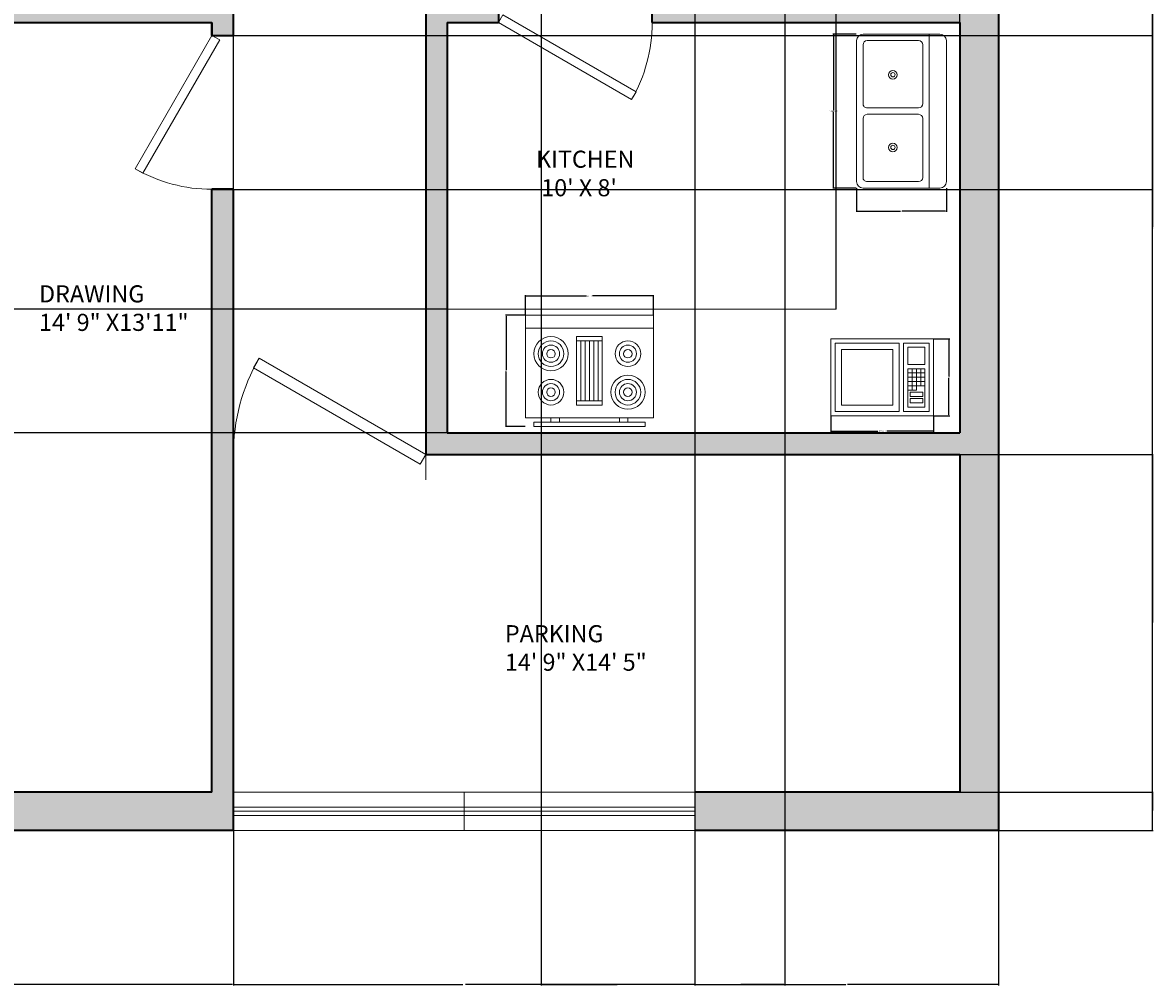
# Model space of a CAD drawing. Units: inches. Extents: x -29 to 404, y -32 to 761.
# Tile 2 of 5: x 139 to 404, y -32 to 193. Entities that reach past the tile are written whole.
import ezdxf

# ---------------------------------------------------------------- set-up
doc = ezdxf.new("R2010")
doc.units = ezdxf.units.IN
doc.header["$MEASUREMENT"] = 0
for name, color, linetype, lineweight in [('A-ANNO-DIMS', 2, 'Continuous', 18), ('A-AREA-IDEN', 7, 'Continuous', 18), ('A-EQPM', 8, 'Continuous', 18), ('A-FLOR-CASE', 8, 'Continuous', 20), ('A-FLOR-FIXT', 9, 'Continuous', 18), ('A-WALL', 7, 'Continuous', 35), ('doors', 40, 'Continuous', 20)]:
    doc.layers.add(name, color=color, linetype=linetype, lineweight=lineweight)
doc.layers.add('A-WALL-PATT', color=251, linetype='Continuous', lineweight=13, true_color=0x636466)
doc.styles.get("Standard").update_dxf_attribs({"font": 'arial.ttf'})
doc.dimstyles.get("Standard").update_dxf_attribs({"dimtxt": 0.18, "dimasz": 0.18, "dimexe": 0.18, "dimexo": 0.0625, "dimgap": 0.09, "dimtad": 0, "dimtih": 1, "dimtoh": 1, "dimdec": 4, "dimzin": 0, "dimdsep": 46, "dimtxsty": 'Standard', "dimcen": 0.09, "dimadec": 0, "dimazin": 0, "dimtfac": 1, "dimtdec": 4, "dimtofl": 0, "dimtmove": 0, "dimatfit": 3, "dimfxl": 1, "dimtolj": 1, "dimtzin": 0, "dimarcsym": 0})

# ---------------------------------------------------------------- blocks, each defined once
blk = doc.blocks.new('Range-Oven - 30 in top')
for p, q in [((0, -3), (30, -3)), ((12, -6), (18, -6)), ((13, -20), (13, -6)), ((14, -6), (14, -20)), ((15, -20), (15, -6)), ((16, -6), (16, -20)), ((17, -20), (17, -6)), ((18, -20), (12, -20)), ((6, -24), (6, -25)), ((8, -25), (8, -24)), ((22, -25), (22, -24)), ((24, -24), (24, -25))]:
    blk.add_line(p, q)
for points in [[(0, -24), (0, 0), (30, 0), (30, -24)], [(12, -21), (12, -5), (18, -5), (18, -21)], [(2, -26), (2, -25), (28, -25), (28, -26)]]:
    blk.add_lwpolyline(points, close=True)
for centre, radius in [((6, -9), 4), ((6, -9), 3), ((6, -9), 2), ((24, -9), 3), ((24, -9), 2), ((6, -9), 1), ((24, -9), 1), ((6, -18), 3), ((24, -18), 4), ((24, -18), 3), ((6, -18), 2), ((6, -18), 1), ((24, -18), 2), ((24, -18), 1)]:
    blk.add_circle(centre, radius)
blk = doc.blocks.new('Sink-double - 36 in top')
for p, q in [((-18, -4), (18, -4)), ((-0.75, -18.5), (-0.75, -6.5)), ((0.75, -6.5), (0.75, -18.5))]:
    blk.add_line(p, q)
for points in [[(-16.5, 0), (16.5, 0)], [(-18, -19.5), (-18, -1.5)], [(18, -1.5), (18, -19.5)], [(-16.5, -18.5), (-16.5, -6.5)], [(-15.5, -5.5), (-1.75, -5.5)], [(1.75, -5.5), (15.5, -5.5)], [(16.5, -6.5), (16.5, -18.5)], [(16.5, -21), (-16.5, -21)], [(-1.75, -19.5), (-15.5, -19.5)], [(15.5, -19.5), (1.75, -19.5)]]:
    blk.add_lwpolyline(points)
for centre, radius in [((-8.5, -12.5), 1), ((-8.5, -12.5), 0.5), ((8.5, -12.5), 1), ((8.5, -12.5), 0.5)]:
    blk.add_circle(centre, radius)
for centre, radius, start, end in [((-16.5, -1.5), 1.5, 90, 180), ((16.5, -1.5), 1.5, 0, 90), ((-15.5, -6.5), 1, 90, 180), ((-1.75, -6.5), 1, 0, 90), ((1.75, -6.5), 1, 90, 180), ((15.5, -6.5), 1, 0, 90), ((-15.5, -18.5), 1, 180, 270), ((-1.75, -18.5), 1, 270, 0), ((1.75, -18.5), 1, 180, 270), ((15.5, -18.5), 1, 270, 0), ((-16.5, -19.5), 1.5, 180, 270), ((16.5, -19.5), 1.5, 270, 0)]:
    blk.add_arc(centre, radius, start, end)
blk = doc.blocks.new('Microwave')
for p, q in [((19, 7), (19, 11)), ((20, 11), (20, 7)), ((21, 7), (21, 11)), ((18, 10), (22, 10)), ((22, 9), (18, 9)), ((18, 8), (22, 8)), ((22, 7), (18, 7)), ((20, 6), (18, 6)), ((19, 6), (19, 7)), ((20, 7), (20, 6))]:
    blk.add_line(p, q)
for points in [[(0, 0), (0, 18), (24, 18), (24, 0)], [(1, 1), (1, 17), (16, 17), (16, 1)], [(17, 1), (17, 17), (23, 17), (23, 1)], [(18, 12), (18, 16), (22, 16), (22, 12)], [(2.5, 2.5), (2.5, 15.5), (14.5, 15.5), (14.5, 2.5)], [(18, 2), (18, 11), (22, 11), (22, 2)], [(18.5, 4.5), (18.5, 5.5), (21.5, 5.5), (21.5, 4.5)], [(18.5, 3), (18.5, 4), (21.5, 4), (21.5, 3)]]:
    blk.add_lwpolyline(points, close=True)
blk = doc.blocks.new('*U7')
for p, q in [((0, 0), (0, 100)), ((750, 0), (750, 100))]:
    blk.add_line(p, q)
blk.add_lwpolyline([(0, 0), (649.5, -375), (671.4, -337.1), (21.9, 37.9)], close=True)
blk.add_arc((0, 0), 750, 330, 0)
blk = doc.blocks.new('*D25')
at = {"layer": 'A-ANNO-DIMS', "color": 0, "lineweight": -2, "transparency": 16777216}
for p, q in [((256.99, 125.04), (256.99, 129.66)), ((286.99, 125.04), (286.99, 129.66)), ((257.17, 129.48), (271.3, 129.48)), ((286.81, 129.48), (272.69, 129.48))]:
    blk.add_line(p, q, dxfattribs=at)
at = {"layer": 'A-ANNO-DIMS', "color": 0, "transparency": 16777216}
for points in [[(257.17, 129.51), (257.17, 129.45), (256.99, 129.48)], [(286.81, 129.51), (286.81, 129.45), (286.99, 129.48)]]:
    blk.add_solid(points, dxfattribs=at)
at = {"layer": 'Defpoints', "color": 0, "transparency": 16777216}
for p in [(286.99, 129.48), (256.99, 124.98), (286.99, 124.98)]:
    blk.add_point(p, dxfattribs=at)
at = {"layer": 'A-ANNO-DIMS', "color": 0, "transparency": 16777216, "insert": (271.99, 129.48), "char_height": 0.18, "attachment_point": 5}
blk.add_mtext('\\A1;RANGE 30', dxfattribs=at)
blk = doc.blocks.new('*D26')
at = {"layer": 'A-ANNO-DIMS', "color": 0, "lineweight": -2, "transparency": 16777216}
for p, q in [((256.93, 124.98), (252.31, 124.98)), ((252.49, 124.8), (252.49, 112.16)), ((252.49, 99.16), (252.49, 111.8)), ((256.93, 98.98), (252.31, 98.98))]:
    blk.add_line(p, q, dxfattribs=at)
at = {"layer": 'A-ANNO-DIMS', "color": 0, "transparency": 16777216}
for points in [[(252.46, 124.8), (252.52, 124.8), (252.49, 124.98)], [(252.46, 99.16), (252.52, 99.16), (252.49, 98.98)]]:
    blk.add_solid(points, dxfattribs=at)
at = {"layer": 'Defpoints', "color": 0, "transparency": 16777216}
for p in [(252.49, 124.98), (256.99, 124.98), (256.99, 98.98)]:
    blk.add_point(p, dxfattribs=at)
at = {"layer": 'A-ANNO-DIMS', "color": 0, "transparency": 16777216, "insert": (252.49, 111.98), "char_height": 0.18, "attachment_point": 5}
blk.add_mtext('\\A1;26', dxfattribs=at)
blk = doc.blocks.new('*D27')
at = {"layer": 'A-ANNO-DIMS', "color": 0, "lineweight": -2, "transparency": 16777216}
for p, q in [((334.43, 190.73), (328.91, 190.73)), ((329.09, 190.55), (329.09, 172.91)), ((329.09, 154.91), (329.09, 172.55)), ((334.43, 154.73), (328.91, 154.73))]:
    blk.add_line(p, q, dxfattribs=at)
at = {"layer": 'A-ANNO-DIMS', "color": 0, "transparency": 16777216}
for points in [[(329.06, 190.55), (329.12, 190.55), (329.09, 190.73)], [(329.06, 154.91), (329.12, 154.91), (329.09, 154.73)]]:
    blk.add_solid(points, dxfattribs=at)
at = {"layer": 'Defpoints', "color": 0, "transparency": 16777216}
for p in [(334.49, 190.73), (329.09, 154.73), (334.49, 154.73)]:
    blk.add_point(p, dxfattribs=at)
at = {"layer": 'A-ANNO-DIMS', "color": 0, "transparency": 16777216, "insert": (329.09, 172.73), "char_height": 0.18, "attachment_point": 5}
blk.add_mtext('\\A1;DOUBLE SINK 36', dxfattribs=at)
blk = doc.blocks.new('*D28')
at = {"layer": 'A-ANNO-DIMS', "color": 0, "lineweight": -2, "transparency": 16777216}
for p, q in [((334.49, 154.67), (334.49, 149.15)), ((355.49, 154.67), (355.49, 149.15)), ((334.67, 149.33), (344.79, 149.33)), ((355.31, 149.33), (345.19, 149.33))]:
    blk.add_line(p, q, dxfattribs=at)
at = {"layer": 'A-ANNO-DIMS', "color": 0, "transparency": 16777216}
for points in [[(334.67, 149.36), (334.67, 149.3), (334.49, 149.33)], [(355.31, 149.36), (355.31, 149.3), (355.49, 149.33)]]:
    blk.add_solid(points, dxfattribs=at)
at = {"layer": 'Defpoints', "color": 0, "transparency": 16777216}
for p in [(334.49, 154.73), (355.49, 154.73), (355.49, 149.33)]:
    blk.add_point(p, dxfattribs=at)
at = {"layer": 'A-ANNO-DIMS', "color": 0, "transparency": 16777216, "insert": (344.99, 149.33), "char_height": 0.18, "attachment_point": 5}
blk.add_mtext('\\A1;21', dxfattribs=at)
blk = doc.blocks.new('*D29')
at = {"layer": 'A-ANNO-DIMS', "color": 0, "lineweight": -2, "transparency": 16777216}
for p, q in [((328.49, 101.42), (328.49, 97.7)), ((352.49, 101.42), (352.49, 97.7)), ((328.67, 97.88), (339.45, 97.88)), ((352.31, 97.88), (341.53, 97.88))]:
    blk.add_line(p, q, dxfattribs=at)
at = {"layer": 'A-ANNO-DIMS', "color": 0, "transparency": 16777216}
for points in [[(328.67, 97.91), (328.67, 97.85), (328.49, 97.88)], [(352.31, 97.91), (352.31, 97.85), (352.49, 97.88)]]:
    blk.add_solid(points, dxfattribs=at)
at = {"layer": 'Defpoints', "color": 0, "transparency": 16777216}
for p in [(328.49, 101.48), (352.49, 101.48), (352.49, 97.88)]:
    blk.add_point(p, dxfattribs=at)
at = {"layer": 'A-ANNO-DIMS', "color": 0, "transparency": 16777216, "insert": (340.49, 97.88), "char_height": 0.18, "attachment_point": 5}
blk.add_mtext('\\A1;MICROWAVE 24', dxfattribs=at)
blk = doc.blocks.new('*D30')
at = {"layer": 'A-ANNO-DIMS', "color": 0, "lineweight": -2, "transparency": 16777216}
for p, q in [((352.55, 119.48), (356.27, 119.48)), ((356.09, 119.3), (356.09, 110.66)), ((356.09, 101.66), (356.09, 110.3)), ((352.55, 101.48), (356.27, 101.48))]:
    blk.add_line(p, q, dxfattribs=at)
at = {"layer": 'A-ANNO-DIMS', "color": 0, "transparency": 16777216}
for points in [[(356.06, 119.3), (356.12, 119.3), (356.09, 119.48)], [(356.06, 101.66), (356.12, 101.66), (356.09, 101.48)]]:
    blk.add_solid(points, dxfattribs=at)
at = {"layer": 'Defpoints', "color": 0, "transparency": 16777216}
for p in [(352.49, 119.48), (356.09, 119.48), (352.49, 101.48)]:
    blk.add_point(p, dxfattribs=at)
at = {"layer": 'A-ANNO-DIMS', "color": 0, "transparency": 16777216, "insert": (356.09, 110.48), "char_height": 0.18, "attachment_point": 5}
blk.add_mtext('\\A1;18', dxfattribs=at)
blk = doc.blocks.new('*D32')
at = {"layer": 'A-ANNO-DIMS', "color": 0, "lineweight": -2, "transparency": 16777216}
for p, q in [((367.74, 724.43), (403.91, 724.43)), ((403.73, 724.25), (403.73, 364.62)), ((403.73, 4.61), (403.73, 364.25)), ((367.74, 4.43), (403.91, 4.43))]:
    blk.add_line(p, q, dxfattribs=at)
at = {"layer": 'A-ANNO-DIMS', "color": 0, "transparency": 16777216}
for points in [[(403.7, 724.25), (403.76, 724.25), (403.73, 724.43)], [(403.7, 4.61), (403.76, 4.61), (403.73, 4.43)]]:
    blk.add_solid(points, dxfattribs=at)
at = {"layer": 'Defpoints', "color": 0, "transparency": 16777216}
for p in [(367.68, 724.43), (403.73, 724.43), (367.68, 4.43)]:
    blk.add_point(p, dxfattribs=at)
at = {"layer": 'A-ANNO-DIMS', "color": 0, "transparency": 16777216, "insert": (403.73, 364.43), "char_height": 0.18, "attachment_point": 5}
blk.add_mtext('\\A1;720', dxfattribs=at)
blk = doc.blocks.new('*D38')
at = {"layer": 'A-ANNO-DIMS', "color": 0, "lineweight": -2, "transparency": 16777216}
for p, q in [((7.68, 4.37), (7.68, -31.8)), ((188.68, 4.37), (188.68, -31.8)), ((7.86, -31.62), (97.92, -31.62)), ((188.5, -31.62), (98.44, -31.62))]:
    blk.add_line(p, q, dxfattribs=at)
at = {"layer": 'A-ANNO-DIMS', "color": 0, "transparency": 16777216}
for points in [[(7.86, -31.59), (7.86, -31.65), (7.68, -31.62)], [(188.5, -31.59), (188.5, -31.65), (188.68, -31.62)]]:
    blk.add_solid(points, dxfattribs=at)
at = {"layer": 'Defpoints', "color": 0, "transparency": 16777216}
for p in [(7.68, 4.43), (188.68, 4.43), (188.68, -31.62)]:
    blk.add_point(p, dxfattribs=at)
at = {"layer": 'A-ANNO-DIMS', "color": 0, "transparency": 16777216, "insert": (98.18, -31.62), "char_height": 0.18, "attachment_point": 5}
blk.add_mtext('\\A1;181', dxfattribs=at)
blk = doc.blocks.new('*D39')
at = {"layer": 'A-ANNO-DIMS', "color": 0, "lineweight": -2, "transparency": 16777216}
for p, q in [((188.68, 4.37), (188.68, -31.8)), ((296.68, 4.37), (296.68, -31.8)), ((188.86, -31.62), (242.4, -31.62)), ((296.5, -31.62), (242.96, -31.62))]:
    blk.add_line(p, q, dxfattribs=at)
at = {"layer": 'A-ANNO-DIMS', "color": 0, "transparency": 16777216}
for points in [[(188.86, -31.59), (188.86, -31.65), (188.68, -31.62)], [(296.5, -31.59), (296.5, -31.65), (296.68, -31.62)]]:
    blk.add_solid(points, dxfattribs=at)
at = {"layer": 'Defpoints', "color": 0, "transparency": 16777216}
for p in [(188.68, 4.43), (296.68, 4.43), (296.68, -31.62)]:
    blk.add_point(p, dxfattribs=at)
at = {"layer": 'A-ANNO-DIMS', "color": 0, "transparency": 16777216, "insert": (242.68, -31.62), "char_height": 0.18, "attachment_point": 5}
blk.add_mtext('\\A1;108', dxfattribs=at)
blk = doc.blocks.new('*D40')
at = {"layer": 'A-ANNO-DIMS', "color": 0, "lineweight": -2, "transparency": 16777216}
for p, q in [((296.68, 4.37), (296.68, -31.8)), ((367.68, 4.37), (367.68, -31.8)), ((296.86, -31.62), (331.98, -31.62)), ((367.5, -31.62), (332.38, -31.62))]:
    blk.add_line(p, q, dxfattribs=at)
at = {"layer": 'A-ANNO-DIMS', "color": 0, "transparency": 16777216}
for points in [[(296.86, -31.59), (296.86, -31.65), (296.68, -31.62)], [(367.5, -31.59), (367.5, -31.65), (367.68, -31.62)]]:
    blk.add_solid(points, dxfattribs=at)
at = {"layer": 'Defpoints', "color": 0, "transparency": 16777216}
for p in [(296.68, 4.43), (367.68, 4.43), (367.68, -31.62)]:
    blk.add_point(p, dxfattribs=at)
at = {"layer": 'A-ANNO-DIMS', "color": 0, "transparency": 16777216, "insert": (332.18, -31.62), "char_height": 0.18, "attachment_point": 5}
blk.add_mtext('\\A1;71', dxfattribs=at)
blk = doc.blocks.new('*D43')
at = {"layer": 'A-ANNO-DIMS', "color": 0, "lineweight": -2, "transparency": 16777216}
for p, q in [((358.74, 92.43), (403.91, 92.43)), ((403.73, 92.25), (403.73, 53.12)), ((403.73, 13.61), (403.73, 52.75)), ((358.74, 13.43), (403.91, 13.43))]:
    blk.add_line(p, q, dxfattribs=at)
at = {"layer": 'A-ANNO-DIMS', "color": 0, "transparency": 16777216}
for points in [[(403.7, 92.25), (403.76, 92.25), (403.73, 92.43)], [(403.7, 13.61), (403.76, 13.61), (403.73, 13.43)]]:
    blk.add_solid(points, dxfattribs=at)
at = {"layer": 'Defpoints', "color": 0, "transparency": 16777216}
for p in [(358.68, 92.43), (403.73, 92.43), (358.68, 13.43)]:
    blk.add_point(p, dxfattribs=at)
at = {"layer": 'A-ANNO-DIMS', "color": 0, "transparency": 16777216, "insert": (403.73, 52.93), "char_height": 0.18, "attachment_point": 5}
blk.add_mtext('\\A1;79', dxfattribs=at)
blk = doc.blocks.new('*D44')
at = {"layer": 'A-ANNO-DIMS', "color": 0, "lineweight": -2, "transparency": 16777216}
for p, q in [((188.68, 92.5), (188.68, 760.66)), ((188.86, 760.48), (210.95, 760.48)), ((233.5, 760.48), (211.4, 760.48)), ((233.68, 92.5), (233.68, 760.66))]:
    blk.add_line(p, q, dxfattribs=at)
at = {"layer": 'A-ANNO-DIMS', "color": 0, "transparency": 16777216}
for points in [[(188.86, 760.51), (188.86, 760.45), (188.68, 760.48)], [(233.5, 760.51), (233.5, 760.45), (233.68, 760.48)]]:
    blk.add_solid(points, dxfattribs=at)
at = {"layer": 'Defpoints', "color": 0, "transparency": 16777216}
for p in [(233.68, 760.48), (188.68, 92.43), (233.68, 92.43)]:
    blk.add_point(p, dxfattribs=at)
at = {"layer": 'A-ANNO-DIMS', "color": 0, "transparency": 16777216, "insert": (211.18, 760.48), "char_height": 0.18, "attachment_point": 5}
blk.add_mtext('\\A1;45', dxfattribs=at)
blk = doc.blocks.new('*D45')
at = {"layer": 'A-ANNO-DIMS', "color": 0, "lineweight": -2, "transparency": 16777216}
for p, q in [((329.68, 126.5), (329.68, 760.66)), ((329.86, 760.48), (343.96, 760.48)), ((358.5, 760.48), (344.4, 760.48)), ((358.68, 97.5), (358.68, 760.66))]:
    blk.add_line(p, q, dxfattribs=at)
at = {"layer": 'A-ANNO-DIMS', "color": 0, "transparency": 16777216}
for points in [[(329.86, 760.51), (329.86, 760.45), (329.68, 760.48)], [(358.5, 760.51), (358.5, 760.45), (358.68, 760.48)]]:
    blk.add_solid(points, dxfattribs=at)
at = {"layer": 'Defpoints', "color": 0, "transparency": 16777216}
for p in [(358.68, 760.48), (329.68, 126.43), (358.68, 97.43)]:
    blk.add_point(p, dxfattribs=at)
at = {"layer": 'A-ANNO-DIMS', "color": 0, "transparency": 16777216, "insert": (344.18, 760.48), "char_height": 0.18, "attachment_point": 5}
blk.add_mtext('\\A1;29', dxfattribs=at)
blk = doc.blocks.new('*D46')
at = {"layer": 'A-ANNO-DIMS', "color": 0, "lineweight": -2, "transparency": 16777216}
for p, q in [((238.62, 126.43), (-28.55, 126.43)), ((-28.37, 126.25), (-28.37, 112.12)), ((-28.37, 97.61), (-28.37, 111.75)), ((238.62, 97.43), (-28.55, 97.43))]:
    blk.add_line(p, q, dxfattribs=at)
at = {"layer": 'A-ANNO-DIMS', "color": 0, "transparency": 16777216}
for points in [[(-28.4, 126.25), (-28.34, 126.25), (-28.37, 126.43)], [(-28.4, 97.61), (-28.34, 97.61), (-28.37, 97.43)]]:
    blk.add_solid(points, dxfattribs=at)
at = {"layer": 'Defpoints', "color": 0, "transparency": 16777216}
for p in [(-28.37, 126.43), (238.68, 126.43), (238.68, 97.43)]:
    blk.add_point(p, dxfattribs=at)
at = {"layer": 'A-ANNO-DIMS', "color": 0, "transparency": 16777216, "insert": (-28.37, 111.93), "char_height": 0.18, "attachment_point": 5}
blk.add_mtext('\\A1;29', dxfattribs=at)
blk = doc.blocks.new('*D47')
at = {"layer": 'A-ANNO-DIMS', "color": 0, "lineweight": -2, "transparency": 16777216}
for p, q in [((183.74, 190.43), (403.91, 190.43)), ((403.73, 190.25), (403.73, 172.62)), ((403.73, 154.61), (403.73, 172.25)), ((183.74, 154.43), (403.91, 154.43))]:
    blk.add_line(p, q, dxfattribs=at)
at = {"layer": 'A-ANNO-DIMS', "color": 0, "transparency": 16777216}
for points in [[(403.7, 190.25), (403.76, 190.25), (403.73, 190.43)], [(403.7, 154.61), (403.76, 154.61), (403.73, 154.43)]]:
    blk.add_solid(points, dxfattribs=at)
at = {"layer": 'Defpoints', "color": 0, "transparency": 16777216}
for p in [(183.68, 190.43), (403.73, 190.43), (183.68, 154.43)]:
    blk.add_point(p, dxfattribs=at)
at = {"layer": 'A-ANNO-DIMS', "color": 0, "transparency": 16777216, "insert": (403.73, 172.43), "char_height": 0.18, "attachment_point": 5}
blk.add_mtext('\\A1;36', dxfattribs=at)
blk = doc.blocks.new('*D50')
at = {"layer": 'A-ANNO-DIMS', "color": 0, "lineweight": -2, "transparency": 16777216}
for p, q in [((260.68, 466.37), (260.68, -31.8)), ((296.68, 466.37), (296.68, -31.8)), ((260.86, -31.62), (278.46, -31.62)), ((296.5, -31.62), (278.9, -31.62))]:
    blk.add_line(p, q, dxfattribs=at)
at = {"layer": 'A-ANNO-DIMS', "color": 0, "transparency": 16777216}
for points in [[(260.86, -31.59), (260.86, -31.65), (260.68, -31.62)], [(296.5, -31.59), (296.5, -31.65), (296.68, -31.62)]]:
    blk.add_solid(points, dxfattribs=at)
at = {"layer": 'Defpoints', "color": 0, "transparency": 16777216}
for p in [(260.68, 466.43), (296.68, 466.43), (296.68, -31.62)]:
    blk.add_point(p, dxfattribs=at)
at = {"layer": 'A-ANNO-DIMS', "color": 0, "transparency": 16777216, "insert": (278.68, -31.62), "char_height": 0.18, "attachment_point": 5}
blk.add_mtext('\\A1;36', dxfattribs=at)
blk = doc.blocks.new('*D51')
at = {"layer": 'A-ANNO-DIMS', "color": 0, "lineweight": -2, "transparency": 16777216}
for p, q in [((296.68, 471.37), (296.68, -31.8)), ((317.68, 471.37), (317.68, -31.8)), ((296.86, -31.62), (306.97, -31.62)), ((317.5, -31.62), (307.38, -31.62))]:
    blk.add_line(p, q, dxfattribs=at)
at = {"layer": 'A-ANNO-DIMS', "color": 0, "transparency": 16777216}
for points in [[(296.86, -31.59), (296.86, -31.65), (296.68, -31.62)], [(317.5, -31.59), (317.5, -31.65), (317.68, -31.62)]]:
    blk.add_solid(points, dxfattribs=at)
at = {"layer": 'Defpoints', "color": 0, "transparency": 16777216}
for p in [(296.68, 471.43), (317.68, 471.43), (317.68, -31.62)]:
    blk.add_point(p, dxfattribs=at)
at = {"layer": 'A-ANNO-DIMS', "color": 0, "transparency": 16777216, "insert": (307.18, -31.62), "char_height": 0.18, "attachment_point": 5}
blk.add_mtext('\\A1;21', dxfattribs=at)
blk = doc.blocks.new('*D54')
at = {"layer": 'A-ANNO-DIMS', "color": 0, "lineweight": -2, "transparency": 16777216}
for p, q in [((358.74, 13.43), (403.91, 13.43)), ((403.73, 13.25), (403.73, 9.12)), ((403.73, 4.61), (403.73, 8.75)), ((367.74, 4.43), (403.91, 4.43))]:
    blk.add_line(p, q, dxfattribs=at)
at = {"layer": 'A-ANNO-DIMS', "color": 0, "transparency": 16777216}
for points in [[(403.7, 13.25), (403.76, 13.25), (403.73, 13.43)], [(403.7, 4.61), (403.76, 4.61), (403.73, 4.43)]]:
    blk.add_solid(points, dxfattribs=at)
at = {"layer": 'Defpoints', "color": 0, "transparency": 16777216}
for p in [(358.68, 13.43), (367.68, 4.43), (403.73, 4.43)]:
    blk.add_point(p, dxfattribs=at)
at = {"layer": 'A-ANNO-DIMS', "color": 0, "transparency": 16777216, "insert": (403.73, 8.93), "char_height": 0.18, "attachment_point": 5}
blk.add_mtext('\\A1;9', dxfattribs=at)
blk = doc.blocks.new('*D55')
at = {"layer": 'A-ANNO-DIMS', "color": 0, "lineweight": -2, "transparency": 16777216}
for p, q in [((358.74, 198.43), (403.91, 198.43)), ((403.73, 198.25), (403.73, 145.62)), ((403.73, 92.61), (403.73, 145.25)), ((358.74, 92.43), (403.91, 92.43))]:
    blk.add_line(p, q, dxfattribs=at)
at = {"layer": 'A-ANNO-DIMS', "color": 0, "transparency": 16777216}
for points in [[(403.7, 198.25), (403.76, 198.25), (403.73, 198.43)], [(403.7, 92.61), (403.76, 92.61), (403.73, 92.43)]]:
    blk.add_solid(points, dxfattribs=at)
at = {"layer": 'Defpoints', "color": 0, "transparency": 16777216}
for p in [(358.68, 198.43), (403.73, 198.43), (358.68, 92.43)]:
    blk.add_point(p, dxfattribs=at)
at = {"layer": 'A-ANNO-DIMS', "color": 0, "transparency": 16777216, "insert": (403.73, 145.43), "char_height": 0.18, "attachment_point": 5}
blk.add_mtext('\\A1;106', dxfattribs=at)

msp = doc.modelspace()

# ---------------------------------------------------------------- hatches: boundary and pattern name
at = {"layer": 'A-WALL-PATT'}
h = msp.add_hatch(color=256, dxfattribs=at)
h.dxf.hatch_style = 1
h.paths.add_polyline_path([(188.678, 415.434), (183.678, 415.434), (183.678, 287.434), (180.678, 287.434), (180.678, 282.434), (183.678, 282.434), (183.678, 198.434), (57.678, 198.434), (57.678, 282.434), (144.678, 282.434), (144.678, 287.434), (16.678, 287.434), (16.678, 548.434), (144.678, 548.434, -0.1168354), (148.504, 564.585), (148.451, 564.616), (149.501, 566.434), (180.678, 548.434), (180.678, 543.434), (183.678, 543.434), (191.678, 543.434), (191.678, 548.434), (191.678, 553.634), (225.453, 573.134), (226.591, 571.164), (226.533, 571.131, -0.1168354), (230.678, 553.634), (230.678, 548.434), (358.678, 548.434), (358.678, 471.434), (322.678, 471.434), (322.678, 543.434), (358.678, 543.434), (358.678, 548.434), (230.678, 548.434), (230.678, 543.434), (233.678, 543.434), (252.678, 543.434), (252.678, 466.434), (260.678, 466.434), (260.678, 471.434), (257.678, 471.434), (257.678, 543.434), (317.678, 543.434), (317.678, 471.434), (296.678, 471.434), (296.678, 466.434), (358.678, 466.434), (358.678, 198.434), (286.678, 198.434), (286.678, 193.434), (358.678, 193.434), (358.678, 97.434), (238.678, 97.434), (238.678, 193.434), (250.678, 193.434), (250.678, 198.434), (233.678, 198.434), (233.678, 92.434), (358.678, 92.434), (358.678, 13.434), (296.678, 13.434), (296.678, 4.434), (367.678, 4.434), (367.678, 724.434), (7.678, 724.434), (7.678, 4.434), (188.678, 4.434), (188.678, 13.434), (188.678, 154.434), (183.678, 154.434), (183.678, 13.434), (49.651, 13.434), (48.286, 12.069), (46.92, 13.434), (16.678, 13.434), (16.678, 193.434), (183.678, 193.434), (183.678, 190.434), (188.678, 190.434)])
h.paths.add_polyline_path([(52.678, 282.434), (52.678, 198.434), (16.678, 198.434), (16.678, 282.434)], flags=16)

# ---------------------------------------------------------------- linework, layer by layer
at = {"layer": 'A-FLOR-CASE'}
for p, q in [((358.678, 193.434), (329.678, 193.434)), ((329.678, 193.434), (329.678, 126.434)), ((329.678, 126.434), (238.678, 126.434)), ((358.678, 97.434), (358.678, 126.434))]:
    msp.add_line(p, q, dxfattribs=at)
at = {"layer": 'A-WALL'}
for p, q in [((188.678, 190.434), (188.678, 415.434)), ((233.678, 198.434), (233.678, 92.434)), ((250.678, 198.434), (250.678, 193.434)), ((286.678, 193.434), (286.678, 198.434)), ((16.678, 193.434), (183.678, 193.434)), ((183.678, 190.434), (183.678, 193.434)), ((183.678, 193.434), (183.678, 190.434)), ((238.678, 193.434), (250.678, 193.434)), ((238.678, 193.434), (238.678, 97.434)), ((286.678, 193.434), (358.678, 193.434)), ((358.678, 193.434), (358.678, 97.434)), ((183.678, 190.434), (188.678, 190.434)), ((183.678, 13.434), (183.678, 154.434)), ((188.678, 154.434), (183.678, 154.434)), ((188.678, 4.434), (188.678, 154.434)), ((238.678, 97.434), (358.678, 97.434)), ((233.678, 92.434), (358.678, 92.434)), ((358.678, 92.434), (358.678, 13.434)), ((183.678, 13.434), (16.678, 13.434)), ((358.678, 13.434), (296.678, 13.434))]:
    msp.add_line(p, q, dxfattribs=at)
msp.add_lwpolyline([(188.678, 4.434), (7.678, 4.434), (7.678, 724.434), (367.678, 724.434), (367.678, 4.434), (296.678, 4.434)], dxfattribs=at)
at = {"layer": 'doors'}
for p, q in [((296.678, 13.434), (188.678, 13.434)), ((188.678, 13.434), (188.678, 4.434)), ((242.678, 13.434), (242.678, 4.434)), ((296.678, 13.434), (296.678, 4.434)), ((296.678, 4.434), (296.678, 13.434)), ((296.678, 9.934), (188.678, 9.934)), ((296.678, 8.934), (188.678, 8.934)), ((296.678, 7.934), (188.678, 7.934)), ((188.678, 4.434), (296.678, 4.434))]:
    msp.add_line(p, q, dxfattribs=at)

# ---------------------------------------------------------------- block references
at = {"layer": 'A-EQPM'}
for name, p in [('Range-Oven - 30 in top', (256.992, 124.979)), ('Microwave', (328.492, 101.479))]:
    msp.add_blockref(name, p, dxfattribs=at)
at = {"layer": 'A-FLOR-FIXT', "rotation": 270}
msp.add_blockref('Sink-double - 36 in top', (355.492, 172.729), dxfattribs=at)
at = {"layer": 'doors', "xscale": 0.0479999999999998, "yscale": 0.0479999999999998, "zscale": 0.0479999999999998}
msp.add_blockref('*U7', (250.678, 193.434), dxfattribs=at)
at = {"layer": 'doors'}
for p, xscale, yscale, zscale, rotation in [((183.678, 190.434), 0.0479999999999998, 0.0479999999999998, 0.0479999999999998, 270), ((233.678, 92.434), 0.0599999999999998, 0.0599999999999998, 0.0599999999999998, 180)]:
    msp.add_blockref('*U7', p, dxfattribs=dict(at, xscale=xscale, yscale=yscale, zscale=zscale, rotation=rotation))

# ---------------------------------------------------------------- texts
at = {"layer": 'A-AREA-IDEN', "char_height": 4, "attachment_point": 1}
for s, insert in [("KITCHEN\\P 10' X 8'", (259.492, 163.479)), (' DRAWING\\P 14\' 9" X13\'11"', (141.992, 131.979)), (' PARKING\\P 14\' 9" X14\' 5"', (250.992, 52.479))]:
    msp.add_mtext_dynamic_manual_height_columns(s, width=80.5, gutter_width=1, heights=[0], dxfattribs=dict(at, insert=insert))

# ---------------------------------------------------------------- dimensions: what is measured, and where the dimension line sits
at = {"layer": 'A-ANNO-DIMS'}
for base, p1, p2, picture, middle in [((233.678, 760.484), (188.678, 92.434), (233.678, 92.434), '*D44', (211.178, 760.484)), ((358.678, 760.484), (329.678, 126.434), (358.678, 97.434), '*D45', (344.178, 760.484)), ((317.678, -31.616), (296.678, 471.434), (317.678, 471.434), '*D51', (307.178, -31.616)), ((296.678, -31.616), (260.678, 466.434), (296.678, 466.434), '*D50', (278.678, -31.616)), ((355.492, 149.329), (334.492, 154.729), (355.492, 154.729), '*D28', (344.992, 149.329)), ((188.678, -31.616), (7.678, 4.434), (188.678, 4.434), '*D38', (98.178, -31.616)), ((296.678, -31.616), (188.678, 4.434), (296.678, 4.434), '*D39', (242.678, -31.616)), ((367.678, -31.616), (296.678, 4.434), (367.678, 4.434), '*D40', (332.178, -31.616))]:
    dim = msp.add_linear_dim(base=base, p1=p1, p2=p2, dimstyle='Standard', override={"dimdec": 0, "dimlfac": 1, "dimrnd": 0, "dimzin": 0, "dimdsep": 46, "dimlunit": 2}, dxfattribs=at)
    dim.commit()
    dim.dimension.update_dxf_attribs({"geometry": picture, "text_midpoint": middle})
for base, p1, p2, picture, middle in [((403.728, 724.434), (367.678, 4.434), (367.678, 724.434), '*D32', (403.728, 364.434)), ((403.728, 198.434), (358.678, 92.434), (358.678, 198.434), '*D55', (403.728, 145.434)), ((403.728, 190.434), (183.678, 154.434), (183.678, 190.434), '*D47', (403.728, 172.434)), ((-28.372, 126.434), (238.678, 97.434), (238.678, 126.434), '*D46', (-28.372, 111.934)), ((252.492, 124.979), (256.992, 98.979), (256.992, 124.979), '*D26', (252.492, 111.979)), ((356.092, 119.479), (352.492, 101.479), (352.492, 119.479), '*D30', (356.092, 110.479)), ((403.728, 92.434), (358.678, 13.434), (358.678, 92.434), '*D43', (403.728, 52.934)), ((403.728, 4.434), (358.678, 13.434), (367.678, 4.434), '*D54', (403.728, 8.934))]:
    dim = msp.add_linear_dim(base=base, p1=p1, p2=p2, angle=90, dimstyle='Standard', override={"dimdec": 0, "dimlfac": 1, "dimrnd": 0, "dimzin": 0, "dimdsep": 46, "dimlunit": 2}, dxfattribs=at)
    dim.commit()
    dim.dimension.update_dxf_attribs({"geometry": picture, "text_midpoint": middle})
dim = msp.add_linear_dim(base=(329.092, 154.729), p1=(334.492, 190.729), p2=(334.492, 154.729), angle=270, text='DOUBLE SINK <>', dimstyle='Standard', override={"dimdec": 0, "dimlfac": 1, "dimrnd": 0, "dimzin": 0, "dimdsep": 46, "dimlunit": 2}, dxfattribs=at)
dim.commit()
dim.dimension.update_dxf_attribs({"geometry": '*D27', "text_midpoint": (329.092, 172.729)})
for base, p1, p2, text, picture, middle in [((286.992, 129.479), (256.992, 124.979), (286.992, 124.979), 'RANGE <>', '*D25', (271.992, 129.479)), ((352.492, 97.879), (328.492, 101.479), (352.492, 101.479), 'MICROWAVE <>', '*D29', (340.492, 97.879))]:
    dim = msp.add_linear_dim(base=base, p1=p1, p2=p2, text=text, dimstyle='Standard', override={"dimdec": 0, "dimlfac": 1, "dimrnd": 0, "dimzin": 0, "dimdsep": 46, "dimlunit": 2}, dxfattribs=at)
    dim.commit()
    dim.dimension.update_dxf_attribs({"geometry": picture, "text_midpoint": middle})

doc.saveas('drawing.dxf')
